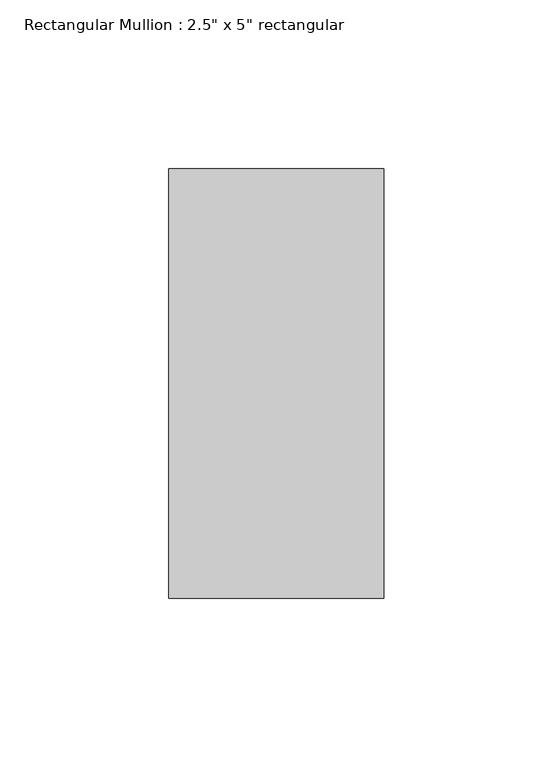
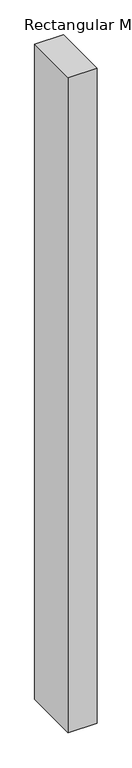
"""IFC4 building model written with IfcOpenShell, lengths in millimetres: member geometry."""

from ifc_helpers import new_model, si_unit, frame, origin, place, context, project, spatial, polyline, outline, extrude, source, transform, mapped, element, save


def member_c9631cd1(model_context):
    return source(origin(), model_context, "Body", "SweptSolid", [
        extrude(outline(polyline([(31.75, 63.5), (31.75, -63.5), (-31.75, -63.5), (-31.75, 63.5), (31.75, 63.5)])), frame((0.0, 0.0, -1521.9137173), z_axis=(0.0, 0.0, 1.0), x_axis=(1.0, 0.0, 0.0)), (0.0, 0.0, 1.0), 1521.9137173),
    ])


if __name__ == "__main__":
    model = new_model("IFC4")
    model_context = context("Model", 3, world=origin())
    ifc_project = project(units=[si_unit("LENGTHUNIT", "METRE", prefix="MILLI")], contexts=[model_context])
    site = spatial("IfcSite", under=ifc_project)
    building = spatial("IfcBuilding", under=site)
    placement = place(None, origin())
    member_shape = member_c9631cd1(model_context)
    element("IfcMember", 1, ObjectType="Rectangular Mullion : 2.5\" x 5\" rectangular", at=placement, inside=building, context=model_context, shape_type="MappedRepresentation", body=[
        mapped(member_shape, transform((0.0, 0.0, 0.0), x_axis=(1.0, 0.0, 0.0), y_axis=(0.0, 1.0, 0.0), z_axis=(0.0, 0.0, 1.0))),
    ])
    save(model, "model.ifc")

# Revit data of these elements
# Type "Rectangular Mullion : 2.5\" x 5\" rectangular"
#   built-in parameter 1007304 = 0.416667 (stored number, unit not read)
#   built-in parameter 1007301 = 0.104167 (stored number, unit not read)
#   built-in parameter 1007300 = 0.104167 (stored number, unit not read)
# Element 1 (IfcMember, "Rectangular Mullion : 2.5\" x 5\" rectangular")
#   Materials on its faces: "Aluminum"
# Materials
#   "Aluminum": class "Metal", colour RGB 247 247 247, transparency 0, Description = "Aluminum 6061", Cost = 0
